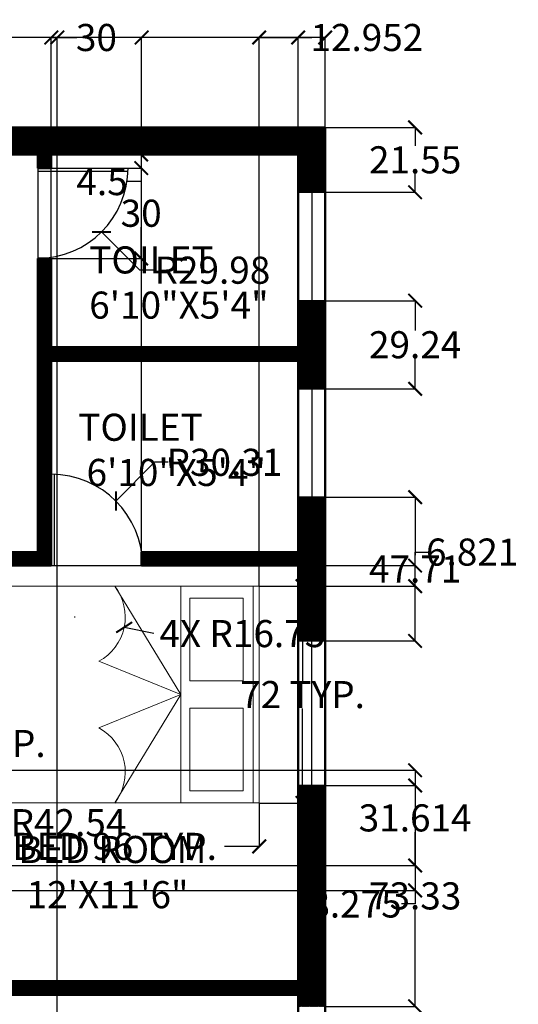
# Model space of a CAD drawing. Units: inches. Extents: x 104 to 466, y -74 to 547.
# Tile 4 of 4: x 300 to 466, y 220 to 547. Entities that reach past the tile are written whole.
import ezdxf

# ---------------------------------------------------------------- set-up
doc = ezdxf.new("R2010")
doc.units = ezdxf.units.IN
doc.header["$MEASUREMENT"] = 0
for name, color, linetype, lineweight in [('A-ANNO-DIMS', 2, 'Continuous', 18), ('A-AREA-IDEN', 7, 'Continuous', 25), ('A-DOOR', 3, 'Continuous', 25), ('A-FURN', 8, 'Continuous', 18), ('A-GLAZ', 4, 'Continuous', 25), ('A-WALL', 7, 'Continuous', 50), ('A-WALL-PATT', 8, 'Continuous', 13)]:
    doc.layers.add(name, color=color, linetype=linetype, lineweight=lineweight)
doc.styles.get("Standard").update_dxf_attribs({"font": 'arial.ttf'})
doc.dimstyles.get("Standard").update_dxf_attribs({"dimtxt": 9, "dimasz": 4.5, "dimexe": 0.18, "dimexo": 0.0625, "dimgap": 0.09, "dimtad": 0, "dimtih": 1, "dimtoh": 1, "dimdec": 1, "dimzin": 0, "dimdsep": 46, "dimlunit": 4, "dimtxsty": 'Standard', "dimblk": 'ARCHTICK', "dimcen": 0.09, "dimadec": 0, "dimazin": 0, "dimtfac": 1, "dimtdec": 1, "dimtofl": 0, "dimtmove": 0, "dimatfit": 3, "dimfxl": 1, "dimtolj": 1, "dimtzin": 0, "dimarcsym": 0})

# ---------------------------------------------------------------- blocks, each defined once
blk = doc.blocks.new('BED-DOUBLE')
for p, q in [((0, 0), (0, 72)), ((0, 72), (96, 72)), ((70, 36), (48, 72)), ((70, 72), (70, 0)), ((94, 72), (94, 0)), ((96, 72), (96, 0)), ((42.75, 47.05), (70, 36)), ((70, 36), (42.75, 24.95)), ((48, 0), (70, 36)), ((96, 0), (0, 0))]:
    blk.add_line(p, q)
for points in [[(90.69, 67.98), (90.69, 40.51), (72.92, 40.51), (72.92, 67.98)], [(90.69, 4.02), (90.69, 31.49), (72.92, 31.49), (72.92, 4.02)]]:
    blk.add_lwpolyline(points, close=True)
for centre, start, end in [((34.78, 61.76), 298.4768, 37.7635), ((34.78, 10.24), 322.2365, 61.5232)]:
    blk.add_arc(centre, 16.73, start, end)
blk = doc.blocks.new('WINDOW-48IN')
for p, q in [((0, 48), (9, 48)), ((0, 0), (0, 48)), ((4.5, 48), (4.5, 0)), ((9, 48), (9, 0)), ((9, 0), (0, 0))]:
    blk.add_line(p, q)
blk = doc.blocks.new('WINDOW-36IN')
for p, q in [((0, 9), (36, 9)), ((0, 0), (0, 9)), ((36, 9), (36, 0)), ((0, 4.5), (36, 4.5)), ((36, 0), (0, 0))]:
    blk.add_line(p, q)
blk = doc.blocks.new('_ArchTick')
at = {"color": 0, "linetype": 'ByBlock', "const_width": 0.15}
blk.add_lwpolyline([(-0.5, -0.5), (0.5, 0.5)], dxfattribs=at)
blk = doc.blocks.new('*D11')
at = {"layer": 'A-ANNO-DIMS', "color": 0, "lineweight": -2, "transparency": 16777216}
for p, q in [((283.63, 286.66), (283.63, 272.14)), ((379.63, 286.66), (379.63, 272.14)), ((283.63, 272.32), (295.16, 272.32)), ((379.63, 272.32), (368.1, 272.32))]:
    blk.add_line(p, q, dxfattribs=at)
at = {"layer": 'Defpoints', "color": 0, "transparency": 16777216}
for p in [(283.63, 286.72), (379.63, 286.72), (379.63, 272.32)]:
    blk.add_point(p, dxfattribs=at)
at = {"layer": 'A-ANNO-DIMS', "color": 0, "lineweight": -2, "transparency": 16777216, "xscale": 4.5, "yscale": 4.5, "zscale": 4.5, "rotation": 180}
blk.add_blockref('_ArchTick', (283.63, 272.32), dxfattribs=at)
at = {"layer": 'A-ANNO-DIMS', "color": 0, "lineweight": -2, "transparency": 16777216, "xscale": 4.5, "yscale": 4.5, "zscale": 4.5}
blk.add_blockref('_ArchTick', (379.63, 272.32), dxfattribs=at)
at = {"layer": 'A-ANNO-DIMS', "color": 0, "transparency": 16777216, "insert": (331.63, 272.32), "char_height": 9, "attachment_point": 5}
blk.add_mtext('\\A1;BED 96 TYP.', dxfattribs=at)
blk = doc.blocks.new('*D12')
at = {"layer": 'A-ANNO-DIMS', "color": 0, "lineweight": -2, "transparency": 16777216}
for p, q in [((379.69, 358.72), (394.21, 358.72)), ((394.03, 358.72), (394.03, 327.34)), ((394.03, 286.72), (394.03, 318.11)), ((379.69, 286.72), (394.21, 286.72))]:
    blk.add_line(p, q, dxfattribs=at)
at = {"layer": 'Defpoints', "color": 0, "transparency": 16777216}
for p in [(379.63, 358.72), (394.03, 358.72), (379.63, 286.72)]:
    blk.add_point(p, dxfattribs=at)
at = {"layer": 'A-ANNO-DIMS', "color": 0, "lineweight": -2, "transparency": 16777216, "xscale": 4.5, "yscale": 4.5, "zscale": 4.5}
for p, rotation in [((394.03, 358.72), 90), ((394.03, 286.72), 270)]:
    blk.add_blockref('_ArchTick', p, dxfattribs=dict(at, rotation=rotation))
at = {"layer": 'A-ANNO-DIMS', "color": 0, "transparency": 16777216, "insert": (394.03, 322.72), "char_height": 9, "attachment_point": 5}
blk.add_mtext('\\A1;72 TYP.', dxfattribs=at)
blk = doc.blocks.new('*D13')
at = {"layer": 'A-ANNO-DIMS', "color": 0, "lineweight": -2, "transparency": 16777216}
for p, q in [((220.21, 305.38), (220.21, 306.66)), ((220.21, 306.48), (227.95, 306.48)), ((227.95, 305.38), (227.95, 306.66)), ((227.95, 306.48), (232.45, 306.48))]:
    blk.add_line(p, q, dxfattribs=at)
at = {"layer": 'Defpoints', "color": 0, "transparency": 16777216}
for p in [(220.21, 305.32), (227.95, 306.48), (227.95, 305.32)]:
    blk.add_point(p, dxfattribs=at)
at = {"layer": 'A-ANNO-DIMS', "color": 0, "lineweight": -2, "transparency": 16777216, "xscale": 4.5, "yscale": 4.5, "zscale": 4.5, "rotation": 180}
blk.add_blockref('_ArchTick', (220.21, 306.48), dxfattribs=at)
at = {"layer": 'A-ANNO-DIMS', "color": 0, "lineweight": -2, "transparency": 16777216, "xscale": 4.5, "yscale": 4.5, "zscale": 4.5}
blk.add_blockref('_ArchTick', (227.95, 306.48), dxfattribs=at)
at = {"layer": 'A-ANNO-DIMS', "color": 0, "transparency": 16777216, "insert": (272.2, 306.48), "char_height": 9, "attachment_point": 5}
blk.add_mtext('\\A1;CHAIR 8 TYP.', dxfattribs=at)
blk = doc.blocks.new('*D17')
at = {"layer": 'A-ANNO-DIMS', "color": 0, "lineweight": -2, "transparency": 16777216}
for p, q in [((159.08, 511.11), (159.08, 541.07)), ((159.08, 540.89), (264.95, 540.89)), ((401.58, 540.89), (295.72, 540.89)), ((401.58, 511.11), (401.58, 541.07))]:
    blk.add_line(p, q, dxfattribs=at)
at = {"layer": 'Defpoints', "color": 0, "transparency": 16777216}
for p in [(401.58, 540.89), (159.08, 511.04), (401.58, 511.04)]:
    blk.add_point(p, dxfattribs=at)
at = {"layer": 'A-ANNO-DIMS', "color": 0, "lineweight": -2, "transparency": 16777216, "xscale": 4.5, "yscale": 4.5, "zscale": 4.5, "rotation": 180}
blk.add_blockref('_ArchTick', (159.08, 540.89), dxfattribs=at)
at = {"layer": 'A-ANNO-DIMS', "color": 0, "lineweight": -2, "transparency": 16777216, "xscale": 4.5, "yscale": 4.5, "zscale": 4.5}
blk.add_blockref('_ArchTick', (401.58, 540.89), dxfattribs=at)
at = {"layer": 'A-ANNO-DIMS', "color": 0, "transparency": 16777216, "insert": (280.33, 540.89), "char_height": 9, "attachment_point": 5}
blk.add_mtext('\\A1;242.5', dxfattribs=at)
blk = doc.blocks.new('*D22')
at = {"layer": 'A-ANNO-DIMS', "color": 0, "lineweight": -2, "transparency": 16777216}
for p, q in [((401.65, 511.04), (431.61, 511.04)), ((431.43, 511.04), (431.43, 504.96)), ((431.43, 489.5), (431.43, 495.59)), ((401.65, 489.5), (431.61, 489.5))]:
    blk.add_line(p, q, dxfattribs=at)
at = {"layer": 'Defpoints', "color": 0, "transparency": 16777216}
for p in [(401.58, 511.04), (401.58, 489.5), (431.43, 489.5)]:
    blk.add_point(p, dxfattribs=at)
at = {"layer": 'A-ANNO-DIMS', "color": 0, "lineweight": -2, "transparency": 16777216, "xscale": 4.5, "yscale": 4.5, "zscale": 4.5}
for p, rotation in [((431.43, 511.04), 90), ((431.43, 489.5), 270)]:
    blk.add_blockref('_ArchTick', p, dxfattribs=dict(at, rotation=rotation))
at = {"layer": 'A-ANNO-DIMS', "color": 0, "transparency": 16777216, "insert": (431.43, 500.27), "char_height": 9, "attachment_point": 5}
blk.add_mtext('\\A1;21.55', dxfattribs=at)
blk = doc.blocks.new('*D23')
at = {"layer": 'A-ANNO-DIMS', "color": 0, "lineweight": -2, "transparency": 16777216}
for p, q in [((401.65, 453.5), (431.61, 453.5)), ((431.43, 453.5), (431.43, 443.56)), ((431.43, 424.25), (431.43, 434.19)), ((401.65, 424.25), (431.61, 424.25))]:
    blk.add_line(p, q, dxfattribs=at)
at = {"layer": 'Defpoints', "color": 0, "transparency": 16777216}
for p in [(401.58, 453.5), (401.58, 424.25), (431.43, 424.25)]:
    blk.add_point(p, dxfattribs=at)
at = {"layer": 'A-ANNO-DIMS', "color": 0, "lineweight": -2, "transparency": 16777216, "xscale": 4.5, "yscale": 4.5, "zscale": 4.5}
for p, rotation in [((431.43, 453.5), 90), ((431.43, 424.25), 270)]:
    blk.add_blockref('_ArchTick', p, dxfattribs=dict(at, rotation=rotation))
at = {"layer": 'A-ANNO-DIMS', "color": 0, "transparency": 16777216, "insert": (431.43, 438.87), "char_height": 9, "attachment_point": 5}
blk.add_mtext('\\A1;29.24', dxfattribs=at)
blk = doc.blocks.new('*D24')
at = {"layer": 'A-ANNO-DIMS', "color": 0, "lineweight": -2, "transparency": 16777216}
for p, q in [((401.65, 388.25), (431.61, 388.25)), ((431.43, 388.25), (431.43, 369.01)), ((431.43, 340.54), (431.43, 359.79)), ((401.65, 340.54), (431.61, 340.54))]:
    blk.add_line(p, q, dxfattribs=at)
at = {"layer": 'Defpoints', "color": 0, "transparency": 16777216}
for p in [(401.58, 388.25), (401.58, 340.54), (431.43, 340.54)]:
    blk.add_point(p, dxfattribs=at)
at = {"layer": 'A-ANNO-DIMS', "color": 0, "lineweight": -2, "transparency": 16777216, "xscale": 4.5, "yscale": 4.5, "zscale": 4.5}
for p, rotation in [((431.43, 388.25), 90), ((431.43, 340.54), 270)]:
    blk.add_blockref('_ArchTick', p, dxfattribs=dict(at, rotation=rotation))
at = {"layer": 'A-ANNO-DIMS', "color": 0, "transparency": 16777216, "insert": (431.43, 364.4), "char_height": 9, "attachment_point": 5}
blk.add_mtext('\\A1;47.71', dxfattribs=at)
blk = doc.blocks.new('*D25')
at = {"layer": 'A-ANNO-DIMS', "color": 0, "lineweight": -2, "transparency": 16777216}
for p, q in [((401.65, 292.54), (431.61, 292.54)), ((431.43, 292.54), (431.43, 260.56)), ((431.43, 219.21), (431.43, 251.19)), ((401.65, 219.21), (431.61, 219.21))]:
    blk.add_line(p, q, dxfattribs=at)
at = {"layer": 'Defpoints', "color": 0, "transparency": 16777216}
for p in [(401.58, 292.54), (401.58, 219.21), (431.43, 219.21)]:
    blk.add_point(p, dxfattribs=at)
at = {"layer": 'A-ANNO-DIMS', "color": 0, "lineweight": -2, "transparency": 16777216, "xscale": 4.5, "yscale": 4.5, "zscale": 4.5}
for p, rotation in [((431.43, 292.54), 90), ((431.43, 219.21), 270)]:
    blk.add_blockref('_ArchTick', p, dxfattribs=dict(at, rotation=rotation))
at = {"layer": 'A-ANNO-DIMS', "color": 0, "transparency": 16777216, "insert": (431.43, 255.88), "char_height": 9, "attachment_point": 5}
blk.add_mtext('\\A1;73.33', dxfattribs=at)
blk = doc.blocks.new('*D37')
at = {"layer": 'A-ANNO-DIMS', "color": 0, "lineweight": -2, "transparency": 16777216}
for p, q in [((264.58, 98.61), (264.58, 541.07)), ((264.58, 540.89), (281.86, 540.89)), ((312.58, 540.89), (295.31, 540.89)), ((312.58, 98.61), (312.58, 541.07))]:
    blk.add_line(p, q, dxfattribs=at)
at = {"layer": 'Defpoints', "color": 0, "transparency": 16777216}
for p in [(312.58, 540.89), (264.58, 98.54), (312.58, 98.54)]:
    blk.add_point(p, dxfattribs=at)
at = {"layer": 'A-ANNO-DIMS', "color": 0, "lineweight": -2, "transparency": 16777216, "xscale": 4.5, "yscale": 4.5, "zscale": 4.5, "rotation": 180}
blk.add_blockref('_ArchTick', (264.58, 540.89), dxfattribs=at)
at = {"layer": 'A-ANNO-DIMS', "color": 0, "lineweight": -2, "transparency": 16777216, "xscale": 4.5, "yscale": 4.5, "zscale": 4.5}
blk.add_blockref('_ArchTick', (312.58, 540.89), dxfattribs=at)
at = {"layer": 'A-ANNO-DIMS', "color": 0, "transparency": 16777216, "insert": (288.58, 540.89), "char_height": 9, "attachment_point": 5}
blk.add_mtext('\\A1;48', dxfattribs=at)
blk = doc.blocks.new('*D41')
at = {"layer": 'A-ANNO-DIMS', "color": 0, "lineweight": -2, "transparency": 16777216}
for p, q in [((228.01, 297.58), (431.61, 297.58)), ((431.43, 297.58), (431.43, 286.47)), ((431.43, 265.97), (431.43, 277.09)), ((228.01, 265.97), (431.61, 265.97))]:
    blk.add_line(p, q, dxfattribs=at)
at = {"layer": 'Defpoints', "color": 0, "transparency": 16777216}
for p in [(227.95, 297.58), (431.43, 297.58), (227.95, 265.97)]:
    blk.add_point(p, dxfattribs=at)
at = {"layer": 'A-ANNO-DIMS', "color": 0, "lineweight": -2, "transparency": 16777216, "xscale": 4.5, "yscale": 4.5, "zscale": 4.5}
for p, rotation in [((431.43, 297.58), 90), ((431.43, 265.97), 270)]:
    blk.add_blockref('_ArchTick', p, dxfattribs=dict(at, rotation=rotation))
at = {"layer": 'A-ANNO-DIMS', "color": 0, "transparency": 16777216, "insert": (431.43, 281.78), "char_height": 9, "attachment_point": 5}
blk.add_mtext('\\A1;31.614', dxfattribs=at)
blk = doc.blocks.new('*D42')
at = {"layer": 'A-ANNO-DIMS', "color": 0, "lineweight": -2, "transparency": 16777216}
for p, q in [((228.01, 265.97), (431.61, 265.97)), ((431.43, 265.97), (431.43, 257.7)), ((220.28, 257.7), (431.61, 257.7)), ((431.43, 257.7), (431.43, 253.19)), ((431.43, 253.19), (426.93, 253.19))]:
    blk.add_line(p, q, dxfattribs=at)
at = {"layer": 'Defpoints', "color": 0, "transparency": 16777216}
for p in [(227.95, 265.97), (220.21, 257.7), (431.43, 257.7)]:
    blk.add_point(p, dxfattribs=at)
at = {"layer": 'A-ANNO-DIMS', "color": 0, "lineweight": -2, "transparency": 16777216, "xscale": 4.5, "yscale": 4.5, "zscale": 4.5}
for p, rotation in [((431.43, 265.97), 90), ((431.43, 257.7), 270)]:
    blk.add_blockref('_ArchTick', p, dxfattribs=dict(at, rotation=rotation))
at = {"layer": 'A-ANNO-DIMS', "color": 0, "transparency": 16777216, "insert": (411.62, 253.19), "char_height": 9, "attachment_point": 5}
blk.add_mtext('\\A1;8.275', dxfattribs=at)
blk = doc.blocks.new('*D47')
at = {"layer": 'A-ANNO-DIMS', "color": 0, "lineweight": -2, "transparency": 16777216}
for p, q in [((310.58, 370.11), (310.58, 541.07)), ((310.58, 540.89), (319.07, 540.89)), ((340.58, 540.89), (332.1, 540.89)), ((340.58, 370.11), (340.58, 541.07))]:
    blk.add_line(p, q, dxfattribs=at)
at = {"layer": 'Defpoints', "color": 0, "transparency": 16777216}
for p in [(340.58, 540.89), (310.58, 370.04), (340.58, 370.04)]:
    blk.add_point(p, dxfattribs=at)
at = {"layer": 'A-ANNO-DIMS', "color": 0, "lineweight": -2, "transparency": 16777216, "xscale": 4.5, "yscale": 4.5, "zscale": 4.5, "rotation": 180}
blk.add_blockref('_ArchTick', (310.58, 540.89), dxfattribs=at)
at = {"layer": 'A-ANNO-DIMS', "color": 0, "lineweight": -2, "transparency": 16777216, "xscale": 4.5, "yscale": 4.5, "zscale": 4.5}
blk.add_blockref('_ArchTick', (340.58, 540.89), dxfattribs=at)
at = {"layer": 'A-ANNO-DIMS', "color": 0, "transparency": 16777216, "insert": (325.58, 540.89), "char_height": 9, "attachment_point": 5}
blk.add_mtext('\\A1;30', dxfattribs=at)
blk = doc.blocks.new('*D48')
at = {"layer": 'A-ANNO-DIMS', "color": 0, "lineweight": -2, "transparency": 16777216}
for p, q in [((310.65, 497.54), (340.61, 497.54)), ((340.43, 497.54), (340.43, 487.23)), ((340.43, 467.54), (340.43, 477.86)), ((310.65, 467.54), (340.61, 467.54))]:
    blk.add_line(p, q, dxfattribs=at)
at = {"layer": 'Defpoints', "color": 0, "transparency": 16777216}
for p in [(310.58, 497.54), (310.58, 467.54), (340.43, 467.54)]:
    blk.add_point(p, dxfattribs=at)
at = {"layer": 'A-ANNO-DIMS', "color": 0, "lineweight": -2, "transparency": 16777216, "xscale": 4.5, "yscale": 4.5, "zscale": 4.5}
for p, rotation in [((340.43, 497.54), 90), ((340.43, 467.54), 270)]:
    blk.add_blockref('_ArchTick', p, dxfattribs=dict(at, rotation=rotation))
at = {"layer": 'A-ANNO-DIMS', "color": 0, "transparency": 16777216, "insert": (340.43, 482.54), "char_height": 9, "attachment_point": 5}
blk.add_mtext('\\A1;30', dxfattribs=at)
blk = doc.blocks.new('*D49')
at = {"layer": 'A-ANNO-DIMS', "color": 0, "lineweight": -2, "transparency": 16777216}
for p, q in [((310.65, 502.04), (340.61, 502.04)), ((340.43, 502.04), (340.43, 497.54)), ((310.65, 497.54), (340.61, 497.54)), ((340.43, 497.54), (340.43, 493.04)), ((340.43, 493.04), (335.93, 493.04))]:
    blk.add_line(p, q, dxfattribs=at)
at = {"layer": 'Defpoints', "color": 0, "transparency": 16777216}
for p in [(310.58, 502.04), (310.58, 497.54), (340.43, 497.54)]:
    blk.add_point(p, dxfattribs=at)
at = {"layer": 'A-ANNO-DIMS', "color": 0, "lineweight": -2, "transparency": 16777216, "xscale": 4.5, "yscale": 4.5, "zscale": 4.5}
for p, rotation in [((340.43, 502.04), 90), ((340.43, 497.54), 270)]:
    blk.add_blockref('_ArchTick', p, dxfattribs=dict(at, rotation=rotation))
at = {"layer": 'A-ANNO-DIMS', "color": 0, "transparency": 16777216, "insert": (327.44, 493.04), "char_height": 9, "attachment_point": 5}
blk.add_mtext('\\A1;4.5', dxfattribs=at)
blk = doc.blocks.new('*D56')
at = {"layer": 'A-ANNO-DIMS', "color": 0, "lineweight": -2, "transparency": 16777216}
for p, q in [((379.63, 358.79), (379.63, 541.07)), ((379.63, 540.89), (392.58, 540.89)), ((392.58, 365.61), (392.58, 541.07)), ((392.58, 540.89), (397.08, 540.89))]:
    blk.add_line(p, q, dxfattribs=at)
at = {"layer": 'Defpoints', "color": 0, "transparency": 16777216}
for p in [(392.58, 540.89), (392.58, 365.54), (379.63, 358.72)]:
    blk.add_point(p, dxfattribs=at)
at = {"layer": 'A-ANNO-DIMS', "color": 0, "lineweight": -2, "transparency": 16777216, "xscale": 4.5, "yscale": 4.5, "zscale": 4.5, "rotation": 180}
blk.add_blockref('_ArchTick', (379.63, 540.89), dxfattribs=at)
at = {"layer": 'A-ANNO-DIMS', "color": 0, "lineweight": -2, "transparency": 16777216, "xscale": 4.5, "yscale": 4.5, "zscale": 4.5}
blk.add_blockref('_ArchTick', (392.58, 540.89), dxfattribs=at)
at = {"layer": 'A-ANNO-DIMS', "color": 0, "transparency": 16777216, "insert": (415.39, 540.89), "char_height": 9, "attachment_point": 5}
blk.add_mtext('\\A1;12.952', dxfattribs=at)
blk = doc.blocks.new('*D57')
at = {"layer": 'A-ANNO-DIMS', "color": 0, "lineweight": -2, "transparency": 16777216}
for p, q in [((431.43, 365.54), (431.43, 370.04)), ((431.43, 370.04), (435.93, 370.04)), ((392.65, 365.54), (431.61, 365.54)), ((431.43, 358.72), (431.43, 365.54)), ((379.69, 358.72), (431.61, 358.72))]:
    blk.add_line(p, q, dxfattribs=at)
at = {"layer": 'Defpoints', "color": 0, "transparency": 16777216}
for p in [(392.58, 365.54), (431.43, 365.54), (379.63, 358.72)]:
    blk.add_point(p, dxfattribs=at)
at = {"layer": 'A-ANNO-DIMS', "color": 0, "lineweight": -2, "transparency": 16777216, "xscale": 4.5, "yscale": 4.5, "zscale": 4.5}
for p, rotation in [((431.43, 365.54), 90), ((431.43, 358.72), 270)]:
    blk.add_blockref('_ArchTick', p, dxfattribs=dict(at, rotation=rotation))
at = {"layer": 'A-ANNO-DIMS', "color": 0, "transparency": 16777216, "insert": (450.37, 370.04), "char_height": 9, "attachment_point": 5}
blk.add_mtext('\\A1;6.821', dxfattribs=at)
blk = doc.blocks.new('*D61')
at = {"layer": 'A-ANNO-DIMS', "color": 0, "lineweight": -2, "transparency": 16777216}
for p, q in [((292.21, 280.18), (274.17, 262.13)), ((296.71, 280.18), (292.21, 280.18)), ((244.08, 231.95), (244.08, 232.13)), ((243.99, 232.04), (244.17, 232.04))]:
    blk.add_line(p, q, dxfattribs=at)
at = {"layer": 'Defpoints', "color": 0, "transparency": 16777216}
for p in [(274.17, 262.13), (244.08, 232.04)]:
    blk.add_point(p, dxfattribs=at)
at = {"layer": 'A-ANNO-DIMS', "color": 0, "lineweight": -2, "transparency": 16777216, "xscale": 4.5, "yscale": 4.5, "zscale": 4.5, "rotation": 225.0001695155098}
blk.add_blockref('_ArchTick', (274.17, 262.13), dxfattribs=at)
at = {"layer": 'A-ANNO-DIMS', "color": 0, "transparency": 16777216, "insert": (316.28, 280.18), "char_height": 9, "attachment_point": 5}
blk.add_mtext('\\A1;R42.54', dxfattribs=at)
blk = doc.blocks.new('*D64')
at = {"layer": 'A-ANNO-DIMS', "color": 0, "lineweight": -2, "transparency": 16777216}
for p, q in [((344.88, 399.84), (332.02, 386.98)), ((349.38, 399.84), (344.88, 399.84)), ((310.49, 365.54), (310.67, 365.54)), ((310.58, 365.45), (310.58, 365.63))]:
    blk.add_line(p, q, dxfattribs=at)
at = {"layer": 'Defpoints', "color": 0, "transparency": 16777216}
for p in [(332.02, 386.98), (310.58, 365.54)]:
    blk.add_point(p, dxfattribs=at)
at = {"layer": 'A-ANNO-DIMS', "color": 0, "lineweight": -2, "transparency": 16777216, "xscale": 4.5, "yscale": 4.5, "zscale": 4.5, "rotation": 225.0002379302577}
blk.add_blockref('_ArchTick', (332.02, 386.98), dxfattribs=at)
at = {"layer": 'A-ANNO-DIMS', "color": 0, "transparency": 16777216, "insert": (368.09, 399.84), "char_height": 9, "attachment_point": 5}
blk.add_mtext('\\A1;R30.31', dxfattribs=at)
blk = doc.blocks.new('*D65')
at = {"layer": 'A-ANNO-DIMS', "color": 0, "lineweight": -2, "transparency": 16777216}
for p, q in [((305.99, 497.54), (306.17, 497.54)), ((306.08, 497.45), (306.08, 497.63)), ((340, 463.63), (327.28, 476.35)), ((344.5, 463.63), (340, 463.63))]:
    blk.add_line(p, q, dxfattribs=at)
at = {"layer": 'Defpoints', "color": 0, "transparency": 16777216}
for p in [(306.08, 497.54), (327.28, 476.35)]:
    blk.add_point(p, dxfattribs=at)
at = {"layer": 'A-ANNO-DIMS', "color": 0, "lineweight": -2, "transparency": 16777216, "xscale": 4.5, "yscale": 4.5, "zscale": 4.5, "rotation": 134.9997918830033}
blk.add_blockref('_ArchTick', (327.28, 476.35), dxfattribs=at)
at = {"layer": 'A-ANNO-DIMS', "color": 0, "transparency": 16777216, "insert": (364.09, 463.63), "char_height": 9, "attachment_point": 5}
blk.add_mtext('\\A1;R29.98', dxfattribs=at)
blk = doc.blocks.new('*D68')
at = {"layer": 'A-ANNO-DIMS', "color": 0, "lineweight": -2, "transparency": 16777216}
for p, q in [((318.32, 348.48), (318.5, 348.48)), ((318.41, 348.39), (318.41, 348.57)), ((344.6, 342.97), (334.78, 345.04))]:
    blk.add_line(p, q, dxfattribs=at)
at = {"layer": 'Defpoints', "color": 0, "transparency": 16777216}
for p in [(318.41, 348.48), (334.78, 345.04)]:
    blk.add_point(p, dxfattribs=at)
at = {"layer": 'A-ANNO-DIMS', "color": 0, "lineweight": -2, "transparency": 16777216, "xscale": 4.5, "yscale": 4.5, "zscale": 4.5, "rotation": 168.1217761042774}
blk.add_blockref('_ArchTick', (334.78, 345.04), dxfattribs=at)
at = {"layer": 'A-ANNO-DIMS', "color": 0, "transparency": 16777216, "insert": (374.03, 342.97), "char_height": 9, "attachment_point": 5}
blk.add_mtext('\\A1;4X R16.73', dxfattribs=at)

msp = doc.modelspace()

# ---------------------------------------------------------------- hatches: boundary and pattern name
at = {"layer": 'A-WALL-PATT'}
h = msp.add_hatch(dxfattribs=at)
h.set_pattern_fill('ANSI31', color=256)
h.set_pattern_definition([(45, (-366.28003, -301.99136), (-0.088388348, 0.088388348), [])])
h.paths.add_polyline_path([(401.5842, 137.0851), (401.5842, 171.2112), (392.5842, 171.2112), (392.5842, 167.545), (332.0842, 167.545), (332.0842, 137.0851), (332.0842, 103.045), (312.5842, 103.045), (312.5842, 98.545), (392.5842, 98.545), (392.5842, -9.455), (392.5842, -30.455), (401.5842, -30.455), (401.5842, 31.361)])
h.paths.add_polyline_path([(392.5842, 103.045), (336.5842, 103.045), (336.5842, 137.0851), (336.5842, 163.045), (392.5842, 163.045), (392.5842, 137.0851)], flags=16)
h.paths.add_polyline_path([(401.5842, 292.5416), (392.5842, 292.5416), (392.5842, 227.545), (248.5842, 227.545), (248.5842, 232.045), (244.0842, 232.045), (244.0842, 223.045), (248.5842, 223.045), (392.5842, 223.045), (392.5842, 219.2112), (401.5842, 219.2112)])
h.paths.add_polyline_path([(401.5842, 388.2533), (392.5842, 388.2533), (392.5842, 370.045), (340.5842, 370.045), (340.5842, 369.865, -0.03576944), (340.8936, 365.545), (392.5842, 365.545), (392.5842, 340.5416), (401.5842, 340.5416)], flags=17)
h.paths.add_polyline_path([(401.5842, 453.4958), (392.5842, 453.4958), (392.5842, 438.045), (310.5842, 438.045), (310.5842, 467.545), (306.0842, 467.545), (306.0842, 370.045), (208.837, 370.045, -0.03088397), (209.1152, 365.545), (244.0842, 365.545), (244.0842, 274.587, -0.0265002), (248.5842, 274.3483), (248.5842, 365.545), (306.0842, 365.545), (310.5842, 365.545), (310.5842, 370.045), (310.5842, 433.545), (392.5842, 433.545), (392.5842, 424.2533), (401.5842, 424.2533)])
h.paths.add_polyline_path([(168.0842, 365.545), (172.5842, 365.545), (172.5842, 370.045), (168.0842, 370.045), (168.0842, 414.671), (159.0842, 414.671), (159.0842, 214.5244), (168.0842, 214.5244)])
h.paths.add_polyline_path([(168.0842, 98.545), (224.0842, 98.545), (224.0842, 103.045), (168.0842, 103.045), (168.0842, 137.0851), (168.0842, 166.5244), (159.0842, 166.5244), (159.0842, 137.0851), (159.0842, 43.0309), (159.0842, -30.455), (168.0842, -30.455), (177.7316, -30.455), (177.7316, -21.455), (168.0842, -21.455), (168.0842, 35.9487)])
h.paths.add_polyline_path([(264.5842, -21.455), (264.5842, 98.545), (264.5842, 103.045), (260.3643, 103.045, -0.03109877), (260.0842, 98.545), (260.0842, -21.455), (248.5842, -21.455), (213.7316, -21.455), (213.7316, -30.455), (248.5842, -30.455), (264.5842, -30.455)])
h.paths.add_polyline_path([(401.5842, 511.045), (159.0842, 511.045), (159.0842, 462.671), (168.0842, 462.671), (168.0842, 502.045), (306.0842, 502.045), (306.0842, 497.545), (310.5842, 497.545), (310.5842, 502.045), (392.5842, 502.045), (392.5842, 489.4958), (401.5842, 489.4958)])

# ---------------------------------------------------------------- linework, layer by layer
at = {"layer": 'A-DOOR'}
for p, q in [((306.0842, 497.545), (336.0634, 497.545)), ((306.0842, 497.545), (306.0842, 467.545)), ((306.0842, 496.545), (336.0467, 496.545)), ((311.5842, 395.8379), (311.5842, 370.045)), ((311.5842, 370.045), (311.5842, 365.545)), ((310.5842, 365.545), (340.5842, 365.545))]:
    msp.add_line(p, q, dxfattribs=at)
for centre, radius, start, end in [((306.0842, 497.545), 29.9793, 270, 0), ((310.5842, 365.545), 30.3094, 0, 90)]:
    msp.add_arc(centre, radius, start, end, dxfattribs=at)
at = {"layer": 'A-WALL'}
for p, q in [((159.0842, 511.045), (401.5842, 511.045)), ((401.5842, 511.045), (401.5842, 137.0851)), ((168.0842, 502.045), (306.0842, 502.045)), ((306.0842, 502.045), (306.0842, 497.545)), ((310.5842, 502.045), (310.5842, 497.545)), ((310.5842, 502.045), (392.5842, 502.045)), ((392.5842, 502.045), (392.5842, 438.045)), ((310.5842, 497.545), (306.0842, 497.545)), ((310.5842, 467.545), (306.0842, 467.545)), ((306.0842, 467.545), (306.0842, 370.045)), ((310.5842, 467.545), (310.5842, 438.045)), ((310.5842, 438.045), (392.5842, 438.045)), ((310.5842, 433.545), (392.5842, 433.545)), ((310.5842, 433.545), (310.5842, 370.045)), ((392.5842, 433.545), (392.5842, 370.045)), ((208.5842, 370.045), (306.0842, 370.045)), ((310.5842, 370.045), (310.5842, 365.545)), ((340.5842, 370.045), (392.5842, 370.045)), ((340.5842, 370.045), (340.5842, 365.545)), ((248.5842, 365.545), (306.0842, 365.545)), ((306.0842, 365.545), (310.5842, 365.545)), ((340.5842, 365.545), (392.5842, 365.545)), ((392.5842, 365.545), (392.5842, 227.545)), ((248.5842, 227.545), (392.5842, 227.545)), ((248.5842, 223.045), (392.5842, 223.045)), ((392.5842, 223.045), (392.5842, 167.545))]:
    msp.add_line(p, q, dxfattribs=at)

# ---------------------------------------------------------------- block references
at = {"layer": 'A-FURN'}
msp.add_blockref('BED-DOUBLE', (283.632, 286.724), dxfattribs=at)
at = {"layer": 'A-GLAZ'}
for name, p, rotation in [('WINDOW-36IN', (392.5842, 489.4954), 269.9999999999999), ('WINDOW-36IN', (392.5842, 424.253), 269.9999999999999), ('WINDOW-48IN', (401.5843, 340.5418), 180)]:
    msp.add_blockref(name, p, dxfattribs=dict(at, rotation=rotation))

# ---------------------------------------------------------------- texts
at = {"layer": 'A-AREA-IDEN', "char_height": 9, "attachment_point": 1}
for s, insert in [(' TOILET\\P 6\'10"X5\'4"', (320.4311, 471.5326)), (' TOILET\\P  6\'10"X5\'4"', (316.7947, 415.9766)), ('BED ROOM\\P 12\'X11\'6"', (299.652, 275.7884))]:
    msp.add_mtext_dynamic_manual_height_columns(s, width=401.09946, gutter_width=1, heights=[0], dxfattribs=dict(at, insert=insert))

# ---------------------------------------------------------------- dimensions: what is measured, and where the dimension line sits
at = {"layer": 'A-ANNO-DIMS'}
for base, p1, p2, override, picture, middle in [((401.5842, 540.895), (159.0842, 511.045), (401.5842, 511.045), {"dimdec": 1, "dimlfac": 1, "dimrnd": 0, "dimzin": 0, "dimdsep": 46, "dimlunit": 2}, '*D17', (280.3342, 540.895)), ((312.5842, 540.895), (264.5842, 98.545), (312.5842, 98.545), {"dimdec": 0, "dimlfac": 1, "dimrnd": 0, "dimzin": 0, "dimdsep": 46, "dimlunit": 2}, '*D37', (288.5842, 540.895)), ((340.5842, 540.895), (310.5842, 370.045), (340.5842, 370.045), {"dimdec": 0, "dimlfac": 1, "dimrnd": 0, "dimzin": 0, "dimdsep": 46, "dimlunit": 2}, '*D47', (325.5842, 540.895)), ((392.5842, 540.895), (379.632, 358.7239), (392.5842, 365.545), {"dimdec": 3, "dimlfac": 1, "dimrnd": 0, "dimzin": 0, "dimdsep": 46, "dimlunit": 2}, '*D56', (415.386, 540.895))]:
    dim = msp.add_linear_dim(base=base, p1=p1, p2=p2, dimstyle='Standard', override=override, dxfattribs=at)
    dim.commit()
    dim.dimension.update_dxf_attribs({"geometry": picture, "text_midpoint": middle})
for base, p1, p2, angle, override, picture, middle in [((431.4342, 489.4958), (401.5842, 511.045), (401.5842, 489.4958), 90, {"dimdec": 2, "dimlfac": 1, "dimrnd": 0, "dimzin": 0, "dimdsep": 46, "dimlunit": 2}, '*D22', (431.4342, 500.2704)), ((340.4342, 497.545), (310.5842, 502.045), (310.5842, 497.545), 270, {"dimdec": 1, "dimlfac": 1, "dimrnd": 0, "dimzin": 0, "dimdsep": 46, "dimlunit": 2}, '*D49', (327.4366, 493.045)), ((340.4342, 467.545), (310.5842, 497.545), (310.5842, 467.545), 270, {"dimdec": 0, "dimlfac": 1, "dimrnd": 0, "dimzin": 0, "dimdsep": 46, "dimlunit": 2}, '*D48', (340.4342, 482.545)), ((431.4342, 424.2533), (401.5842, 453.4958), (401.5842, 424.2533), 90, {"dimdec": 2, "dimlfac": 1, "dimrnd": 0, "dimzin": 0, "dimdsep": 46, "dimlunit": 2}, '*D23', (431.4342, 438.8746)), ((431.4342, 340.5416), (401.5842, 388.2533), (401.5842, 340.5416), 90, {"dimdec": 2, "dimlfac": 1, "dimrnd": 0, "dimzin": 0, "dimdsep": 46, "dimlunit": 2}, '*D24', (431.4342, 364.3975)), ((431.4342, 365.545), (379.632, 358.7239), (392.5842, 365.545), 90, {"dimdec": 3, "dimlfac": 1, "dimrnd": 0, "dimzin": 0, "dimdsep": 46, "dimlunit": 2}, '*D57', (450.3652, 370.045)), ((431.4342, 297.584), (227.951, 265.9698), (227.951, 297.584), 90, {"dimdec": 3, "dimlfac": 1, "dimrnd": 0, "dimzin": 0, "dimdsep": 46, "dimlunit": 2}, '*D41', (431.4342, 281.7769)), ((431.4342, 219.2112), (401.5842, 292.5416), (401.5842, 219.2112), 90, {"dimdec": 2, "dimlfac": 1, "dimrnd": 0, "dimzin": 0, "dimdsep": 46, "dimlunit": 2}, '*D25', (431.4342, 255.8764)), ((431.4342, 257.695), (227.951, 265.9698), (220.2136, 257.695), 90, {"dimdec": 3, "dimlfac": 1, "dimrnd": 0, "dimzin": 0, "dimdsep": 46, "dimlunit": 2}, '*D42', (411.6191, 253.195))]:
    dim = msp.add_linear_dim(base=base, p1=p1, p2=p2, angle=angle, dimstyle='Standard', override=override, dxfattribs=at)
    dim.commit()
    dim.dimension.update_dxf_attribs({"geometry": picture, "text_midpoint": middle})
for center, mpoint, picture, middle in [((306.0842, 497.545), (327.2826, 476.3464), '*D65', (364.0927, 463.6272)), ((310.5842, 365.545), (332.0161, 386.9771), '*D64', (368.0884, 399.8364)), ((244.0842, 232.045), (274.1658, 262.1268), '*D61', (316.2782, 280.1759))]:
    dim = msp.add_radius_dim(center=center, mpoint=mpoint, dimstyle='Standard', override={"dimdec": 2, "dimlfac": 1, "dimrnd": 0, "dimzin": 0, "dimdsep": 46, "dimlunit": 2}, dxfattribs=at)
    dim.commit()
    dim.dimension.update_dxf_attribs({"geometry": picture, "text_midpoint": middle, "dimtype": 164})
dim = msp.add_linear_dim(base=(394.032, 358.7239), p1=(379.632, 286.7239), p2=(379.632, 358.7239), angle=90, text='<> TYP.', dimstyle='Standard', override={"dimdec": 0, "dimlfac": 1, "dimrnd": 0, "dimzin": 0, "dimdsep": 46, "dimlunit": 2}, dxfattribs=at)
dim.commit()
dim.dimension.update_dxf_attribs({"geometry": '*D12', "text_midpoint": (394.032, 322.7239)})
dim = msp.add_radius_dim(center=(318.4073, 348.4793), mpoint=(334.7776, 345.0361), text='4X <>', dimstyle='Standard', override={"dimdec": 2, "dimlfac": 1, "dimrnd": 0, "dimzin": 0, "dimdsep": 46, "dimlunit": 2}, dxfattribs=at)
dim.commit()
dim.dimension.update_dxf_attribs({"geometry": '*D68', "text_midpoint": (344.5998, 342.9701), "dimtype": 164})
for base, p1, p2, text, picture, middle in [((227.951, 306.478), (220.2136, 305.3174), (227.951, 305.3174), 'CHAIR <> TYP.', '*D13', (272.203, 306.478)), ((379.632, 272.3239), (283.632, 286.7239), (379.632, 286.7239), 'BED <> TYP.', '*D11', (331.632, 272.3239))]:
    dim = msp.add_linear_dim(base=base, p1=p1, p2=p2, text=text, dimstyle='Standard', override={"dimdec": 0, "dimlfac": 1, "dimrnd": 0, "dimzin": 0, "dimdsep": 46, "dimlunit": 2}, dxfattribs=at)
    dim.commit()
    dim.dimension.update_dxf_attribs({"geometry": picture, "text_midpoint": middle})

doc.saveas('drawing.dxf')
